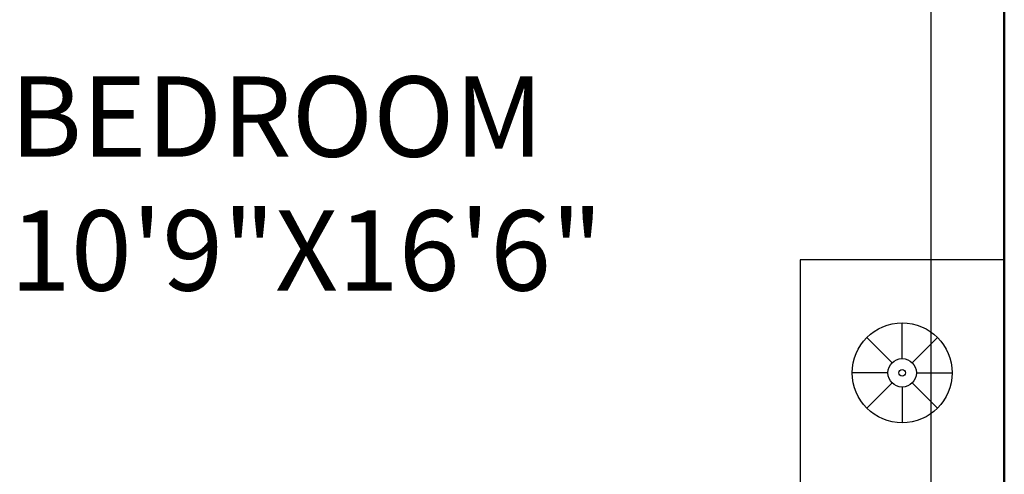
# Model space of a CAD drawing. Units: inches. Extents: x 3064 to 19385, y 846 to 15425.
# Tile 98 of 108: x 7575 to 7661, y 1094 to 1134. Entities that reach past the tile are written whole.
import ezdxf

# ---------------------------------------------------------------- set-up
doc = ezdxf.new("R2010")
doc.units = ezdxf.units.IN
for name, color, linetype, lineweight in [('A-ANNO-DIMS', 2, 'Continuous', 18), ('A-AREA-IDEN', 3, 'Continuous', 18), ('A-FLOR-FIXT', 9, 'Continuous', 18), ('A-WALL', 7, 'Continuous', 50)]:
    doc.layers.add(name, color=color, linetype=linetype, lineweight=lineweight)
doc.layers.add('BLOCK', color=6, linetype='Continuous')
doc.styles.get("Standard").update_dxf_attribs({"font": 'arial.ttf'})
doc.dimstyles.new('ISO-25', dxfattribs={"dimtxt": 9, "dimasz": 2.5, "dimexe": 1.25, "dimexo": 0.625, "dimtad": 1, "dimdec": 1, "dimlunit": 3, "dimtxsty": 'Standard', "dimcen": 2.5, "dimadec": 0, "dimazin": 0, "dimtfac": 1, "dimtdec": 1, "dimtmove": 0, "dimatfit": 3, "dimfxl": 1, "dimarcsym": 0})

# ---------------------------------------------------------------- blocks, each defined once
blk = doc.blocks.new('*D234')
at = {"layer": 'A-ANNO-DIMS', "color": 0, "lineweight": -2, "transparency": 16777216}
for p, q in [((7660.621, 1144.34), (7653.626, 1144.34)), ((7654.876, 984.84), (7654.876, 1141.84)), ((7660.621, 982.34), (7653.626, 982.34))]:
    blk.add_line(p, q, dxfattribs=at)
at = {"layer": 'A-ANNO-DIMS', "color": 0, "transparency": 16777216}
for points in [[(7654.459, 1141.84), (7655.292, 1141.84), (7654.876, 1144.34)], [(7654.459, 984.84), (7655.292, 984.84), (7654.876, 982.34)]]:
    blk.add_solid(points, dxfattribs=at)
at = {"layer": 'Defpoints', "color": 0, "transparency": 16777216}
for p in [(7654.876, 1144.34), (7661.246, 1144.34), (7661.246, 982.34)]:
    blk.add_point(p, dxfattribs=at)
at = {"layer": 'A-ANNO-DIMS', "color": 0, "transparency": 16777216, "insert": (7651.696, 1063.34), "char_height": 5, "attachment_point": 5, "rotation": 90}
blk.add_mtext('13\'-6"', dxfattribs=at)
blk = doc.blocks.new('A$C52E67D0D')
at = {"layer": 'BLOCK'}
for p, q in [((250.5, 1605.5), (250.5, 1684.7)), ((228.3, 1596.3), (172.3, 1652.3)), ((272.7, 1596.3), (328.7, 1652.3)), ((219.1, 1574.1), (139.9, 1574.1)), ((281.9, 1574.1), (361.1, 1574.1)), ((228.3, 1551.9), (172.3, 1495.9)), ((272.7, 1551.9), (328.7, 1495.9)), ((250.5, 1542.8), (250.5, 1463.5))]:
    blk.add_line(p, q, dxfattribs=at)
blk.add_lwpolyline([(501, 1348.6), (501, 1799.6), (0, 1799.6), (0, 1348.6)], close=True, dxfattribs=at)
for radius in [110.6, 31.4, 7.46]:
    blk.add_circle((250.5, 1574.1), radius, dxfattribs=at)

msp = doc.modelspace()

# ---------------------------------------------------------------- linework, layer by layer
at = {"layer": 'A-WALL'}
msp.add_line((7661.246, 1144.34), (7661.246, 982.34), dxfattribs=at)

# ---------------------------------------------------------------- block references
at = {"layer": 'A-FLOR-FIXT', "xscale": 0.039370099999992, "yscale": 0.039370099999992, "zscale": 0.039370099999992, "rotation": 270}
msp.add_blockref('A$C52E67D0D', (7590.38, 1112.592), dxfattribs=at)

# ---------------------------------------------------------------- texts
at = {"layer": 'A-AREA-IDEN', "insert": (7574.659, 1128.57), "char_height": 7, "attachment_point": 1}
msp.add_mtext_dynamic_manual_height_columns('BEDROOM\\P10\'9"X16\'6"', width=67.59241, gutter_width=12.5, heights=[0], dxfattribs=at)

# ---------------------------------------------------------------- dimensions: what is measured, and where the dimension line sits
at = {"layer": 'A-ANNO-DIMS'}
dim = msp.add_linear_dim(base=(7654.876, 1144.34), p1=(7661.246, 982.34), p2=(7661.246, 1144.34), angle=90, dimstyle='ISO-25', override={"dimtxt": 5, "dimclrd": 0, "dimclre": 0, "dimclrt": 0}, dxfattribs=at)
dim.commit()
dim.dimension.update_dxf_attribs({"geometry": '*D234', "text_midpoint": (7651.696, 1063.34)})

doc.saveas('drawing.dxf')
